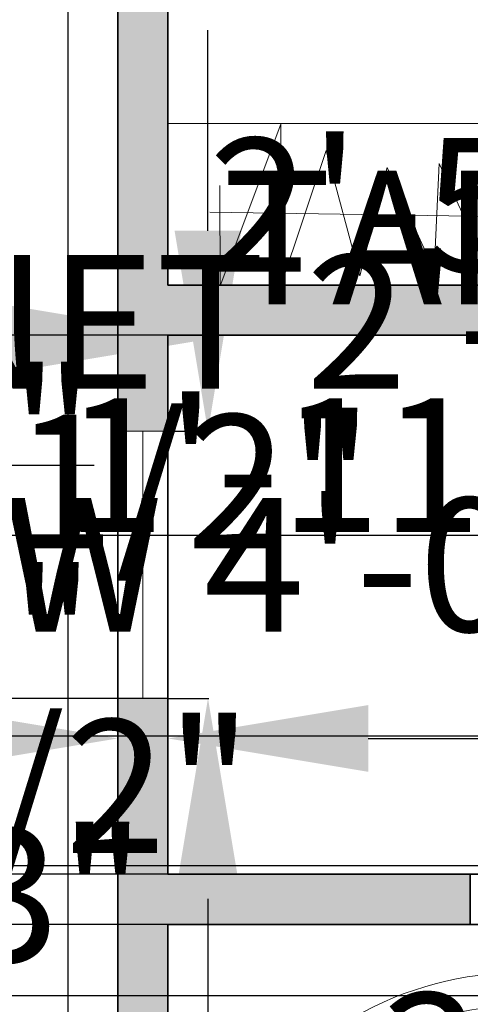
# Model space of a CAD drawing. Units: inches. Extents: x 2838 to 4029, y 1041 to 1915.
# Tile 5 of 16: x 3250 to 3331, y 1377 to 1554. Entities that reach past the tile are written whole.
import ezdxf

# ---------------------------------------------------------------- set-up
doc = ezdxf.new("R2010")
doc.units = ezdxf.units.IN
doc.header["$MEASUREMENT"] = 0
for name, color, linetype, lineweight in [('A-ANNO-DIMS', 2, 'Continuous', 18), ('A-FLOR', 7, 'Continuous', 25), ('A-FLOR-CASE', 8, 'Continuous', 18), ('A-FURN', 8, 'Continuous', 18), ('A-GLAZ', 4, 'Continuous', 18), ('A-WALL', 7, 'Continuous', 35), ('A-WALL-PATT', 252, 'Continuous', 13)]:
    doc.layers.add(name, color=color, linetype=linetype, lineweight=lineweight)
doc.styles.get("Standard").update_dxf_attribs({"font": 'arial.ttf'})
doc.dimstyles.get("Standard").update_dxf_attribs({"dimtxt": 24, "dimasz": 36, "dimexe": 0.18, "dimexo": 0.0625, "dimgap": 0.09, "dimtad": 0, "dimtih": 1, "dimtoh": 1, "dimdec": 0, "dimzin": 0, "dimdsep": 46, "dimlunit": 3, "dimtxsty": 'Standard', "dimcen": 0.09, "dimadec": 0, "dimazin": 0, "dimtfac": 1, "dimtdec": 0, "dimtofl": 0, "dimtmove": 0, "dimatfit": 3, "dimfxl": 1, "dimtolj": 1, "dimtzin": 0, "dimarcsym": 0})

# ---------------------------------------------------------------- blocks, each defined once
blk = doc.blocks.new('Sofa - Roundback Loveseat 5 ft.')
for p, q in [((0, -32.44198), (0, -5.99998)), ((-24, -33.99998), (-24, -11.46958)), ((24.00004, -33.99998), (24.00004, -11.46958)), ((-23.9998, -13.38178), (23.99986, -13.38178)), ((-24, -32.44198), (24.00004, -32.44198))]:
    blk.add_line(p, q)
for points in [[(-24, -33.99998), (-30, -33.99998), (-30, -7.99998)], [(30.00004, -7.99998), (30.00004, -33.99998), (24.00004, -33.99998)]]:
    blk.add_lwpolyline(points)
for centre, radius, start, end in [((0, -60.24998), 60.24998, 60.13715, 119.8628), ((0, -61.38438), 55.38444, 64.32083, 115.6792)]:
    blk.add_arc(centre, radius, start, end)
blk = doc.blocks.new('WIN-48')
blk.add_line((4.5, 48), (4.5, 0))
blk.add_lwpolyline([(0, 48), (9, 48), (9, 0), (0, 0)], close=True)
blk = doc.blocks.new('WARDROBE-RAIL')
for p, q in [((1.86, 0), (12.76, 29.05)), ((12.76, 29.05), (12.76, 0)), ((12.76, 0), (20.9, 24.31)), ((20.9, 24.31), (26.94, 1.83)), ((26.94, 1.83), (31.9, 21.29)), ((31.9, 21.29), (40.3, 2.75)), ((40.3, 2.75), (41.22, 21.97)), ((41.22, 21.97), (49.7, 3.76)), ((1.8, 18), (1.86, 0)), ((49.7, 3.76), (51.56, 19.2)), ((51.56, 19.2), (58.03, 7.54)), ((58.03, 7.54), (58.45, 19.29)), ((58.45, 19.29), (63.49, 12.24)), ((63.49, 12.24), (0, 13.24)), ((0, 13.24), (63.49, 12.24))]:
    blk.add_line(p, q)
blk = doc.blocks.new('*D25')
at = {"layer": 'A-ANNO-DIMS', "color": 0, "lineweight": -2, "transparency": 16777216}
for p, q in [((3283.93, 1516.17), (3283.93, 1552.17)), ((3276.79, 1480.17), (3284.11, 1480.17)), ((3276.79, 1432.17), (3284.11, 1432.17)), ((3283.93, 1396.17), (3283.93, 1360.17))]:
    blk.add_line(p, q, dxfattribs=at)
at = {"layer": 'A-ANNO-DIMS', "color": 0, "transparency": 16777216}
for points in [[(3277.93, 1516.17), (3289.93, 1516.17), (3283.93, 1480.17)], [(3277.93, 1396.17), (3289.93, 1396.17), (3283.93, 1432.17)]]:
    blk.add_solid(points, dxfattribs=at)
at = {"layer": 'Defpoints', "color": 0, "transparency": 16777216}
for p in [(3276.73, 1480.17), (3283.93, 1480.17), (3276.73, 1432.17)]:
    blk.add_point(p, dxfattribs=at)
at = {"layer": 'A-ANNO-DIMS', "color": 0, "transparency": 16777216, "insert": (3283.93, 1456.17), "char_height": 24, "attachment_point": 5}
blk.add_mtext('\\A1;WINDOW 4\'-0" TYP.', dxfattribs=at)
blk = doc.blocks.new('*D26')
at = {"layer": 'A-ANNO-DIMS', "color": 0, "lineweight": -2, "transparency": 16777216}
for p, q in [((3267.73, 1432.1), (3267.73, 1424.79)), ((3276.73, 1432.1), (3276.73, 1424.79)), ((3231.73, 1424.97), (3195.73, 1424.97)), ((3312.73, 1424.97), (3348.73, 1424.97))]:
    blk.add_line(p, q, dxfattribs=at)
at = {"layer": 'A-ANNO-DIMS', "color": 0, "transparency": 16777216}
for points in [[(3231.73, 1430.97), (3231.73, 1418.97), (3267.73, 1424.97)], [(3312.73, 1430.97), (3312.73, 1418.97), (3276.73, 1424.97)]]:
    blk.add_solid(points, dxfattribs=at)
at = {"layer": 'Defpoints', "color": 0, "transparency": 16777216}
for p in [(3267.73, 1432.17), (3276.73, 1432.17), (3276.73, 1424.97)]:
    blk.add_point(p, dxfattribs=at)
at = {"layer": 'A-ANNO-DIMS', "color": 0, "transparency": 16777216, "insert": (3421.97, 1424.97), "char_height": 24, "attachment_point": 5}
blk.add_mtext('\\A1;0\'-9" TYP.', dxfattribs=at)
blk = doc.blocks.new('*D30')
at = {"layer": 'A-ANNO-DIMS', "color": 0, "lineweight": -2, "transparency": 16777216}
for p, q in [((3379.15, 1421.58), (3379.15, 1457.58)), ((3370.21, 1385.58), (3379.33, 1385.58)), ((3370.21, 1348.91), (3379.33, 1348.91)), ((3379.15, 1312.91), (3379.15, 1276.91))]:
    blk.add_line(p, q, dxfattribs=at)
at = {"layer": 'A-ANNO-DIMS', "color": 0, "transparency": 16777216}
for points in [[(3373.15, 1421.58), (3385.15, 1421.58), (3379.15, 1385.58)], [(3373.15, 1312.91), (3385.15, 1312.91), (3379.15, 1348.91)]]:
    blk.add_solid(points, dxfattribs=at)
at = {"layer": 'Defpoints', "color": 0, "transparency": 16777216}
for p in [(3370.15, 1385.58), (3379.15, 1385.58), (3370.15, 1348.91)]:
    blk.add_point(p, dxfattribs=at)
at = {"layer": 'A-ANNO-DIMS', "color": 0, "transparency": 16777216, "insert": (3379.15, 1367.25), "char_height": 24, "attachment_point": 5}
blk.add_mtext('\\A1;3\'-0 1/2"', dxfattribs=at)
blk = doc.blocks.new('*D35')
at = {"layer": 'A-ANNO-DIMS', "color": 0, "lineweight": -2, "transparency": 16777216}
for p, q in [((3480.45, 1632.93), (3480.45, 1668.93)), ((3481.89, 1596.93), (3480.27, 1596.93)), ((3481.89, 1586.93), (3480.27, 1586.93)), ((3480.45, 1550.93), (3480.45, 1514.93)), ((3480.45, 1514.93), (3444.45, 1514.93))]:
    blk.add_line(p, q, dxfattribs=at)
at = {"layer": 'A-ANNO-DIMS', "color": 0, "transparency": 16777216}
for points in [[(3474.45, 1632.93), (3486.45, 1632.93), (3480.45, 1596.93)], [(3474.45, 1550.93), (3486.45, 1550.93), (3480.45, 1586.93)]]:
    blk.add_solid(points, dxfattribs=at)
at = {"layer": 'Defpoints', "color": 0, "transparency": 16777216}
for p in [(3481.95, 1596.93), (3480.45, 1586.93), (3481.95, 1586.93)]:
    blk.add_point(p, dxfattribs=at)
at = {"layer": 'A-ANNO-DIMS', "color": 0, "transparency": 16777216, "insert": (3365.58, 1514.93), "char_height": 24, "attachment_point": 5}
blk.add_mtext('\\A1;TAP 0\'-10"', dxfattribs=at)
blk = doc.blocks.new('*D38')
at = {"layer": 'A-ANNO-DIMS', "color": 0, "lineweight": -2, "transparency": 16777216}
for p, q in [((3368.73, 1671.36), (3368.73, 1707.36)), ((3356.79, 1635.36), (3368.91, 1635.36)), ((3356.79, 1575.36), (3368.91, 1575.36)), ((3368.73, 1539.36), (3368.73, 1503.36))]:
    blk.add_line(p, q, dxfattribs=at)
at = {"layer": 'A-ANNO-DIMS', "color": 0, "transparency": 16777216}
for points in [[(3362.73, 1671.36), (3374.73, 1671.36), (3368.73, 1635.36)], [(3362.73, 1539.36), (3374.73, 1539.36), (3368.73, 1575.36)]]:
    blk.add_solid(points, dxfattribs=at)
at = {"layer": 'Defpoints', "color": 0, "transparency": 16777216}
for p in [(3356.73, 1635.36), (3368.73, 1635.36), (3356.73, 1575.36)]:
    blk.add_point(p, dxfattribs=at)
at = {"layer": 'A-ANNO-DIMS', "color": 0, "transparency": 16777216, "insert": (3368.73, 1605.36), "char_height": 24, "attachment_point": 5}
blk.add_mtext('\\A1;5\'-0" TYP.', dxfattribs=at)
blk = doc.blocks.new('*D41')
at = {"layer": 'A-ANNO-DIMS', "color": 0, "lineweight": -2, "transparency": 16777216}
for p, q in [((3284.24, 1506.2), (3284.24, 1496.56)), ((3347.73, 1506.2), (3347.73, 1496.56)), ((3248.24, 1496.74), (3212.24, 1496.74)), ((3383.73, 1496.74), (3419.73, 1496.74))]:
    blk.add_line(p, q, dxfattribs=at)
at = {"layer": 'A-ANNO-DIMS', "color": 0, "transparency": 16777216}
for points in [[(3248.24, 1502.74), (3248.24, 1490.74), (3284.24, 1496.74)], [(3383.73, 1502.74), (3383.73, 1490.74), (3347.73, 1496.74)]]:
    blk.add_solid(points, dxfattribs=at)
at = {"layer": 'Defpoints', "color": 0, "transparency": 16777216}
for p in [(3284.24, 1506.26), (3347.73, 1506.26), (3347.73, 1496.74)]:
    blk.add_point(p, dxfattribs=at)
at = {"layer": 'A-ANNO-DIMS', "color": 0, "transparency": 16777216, "insert": (3624.81, 1496.74), "char_height": 24, "attachment_point": 5}
blk.add_mtext('\\A1;WARDROBE 5\'-3 1/2" TYP.', dxfattribs=at)
blk = doc.blocks.new('*D42')
at = {"layer": 'A-ANNO-DIMS', "color": 0, "lineweight": -2, "transparency": 16777216}
for p, q in [((3357.26, 1571.32), (3357.26, 1607.32)), ((3347.8, 1535.32), (3357.44, 1535.32)), ((3347.8, 1506.26), (3357.44, 1506.26)), ((3357.26, 1470.26), (3357.26, 1434.26))]:
    blk.add_line(p, q, dxfattribs=at)
at = {"layer": 'A-ANNO-DIMS', "color": 0, "transparency": 16777216}
for points in [[(3351.26, 1571.32), (3363.26, 1571.32), (3357.26, 1535.32)], [(3351.26, 1470.26), (3363.26, 1470.26), (3357.26, 1506.26)]]:
    blk.add_solid(points, dxfattribs=at)
at = {"layer": 'Defpoints', "color": 0, "transparency": 16777216}
for p in [(3347.73, 1535.32), (3357.26, 1535.32), (3347.73, 1506.26)]:
    blk.add_point(p, dxfattribs=at)
at = {"layer": 'A-ANNO-DIMS', "color": 0, "transparency": 16777216, "insert": (3357.26, 1520.79), "char_height": 24, "attachment_point": 5}
blk.add_mtext('\\A1;2\'-5" TYP.', dxfattribs=at)
blk = doc.blocks.new('*D55')
at = {"layer": 'A-ANNO-DIMS', "color": 0, "lineweight": -2, "transparency": 16777216}
for p, q in [((3491.76, 1499.78), (3455.76, 1499.78)), ((3527.76, 1494.67), (3527.76, 1499.96)), ((3562.26, 1494.67), (3562.26, 1499.96)), ((3598.26, 1499.78), (3634.26, 1499.78))]:
    blk.add_line(p, q, dxfattribs=at)
at = {"layer": 'A-ANNO-DIMS', "color": 0, "transparency": 16777216}
for points in [[(3491.76, 1505.78), (3491.76, 1493.78), (3527.76, 1499.78)], [(3598.26, 1505.78), (3598.26, 1493.78), (3562.26, 1499.78)]]:
    blk.add_solid(points, dxfattribs=at)
at = {"layer": 'Defpoints', "color": 0, "transparency": 16777216}
for p in [(3527.76, 1499.78), (3527.76, 1494.6), (3562.26, 1494.6)]:
    blk.add_point(p, dxfattribs=at)
at = {"layer": 'A-ANNO-DIMS', "color": 0, "transparency": 16777216, "insert": (3260.33, 1499.78), "char_height": 24, "attachment_point": 5}
blk.add_mtext('\\A1;BASE CABINET 2\'-10 1/2"', dxfattribs=at)
blk = doc.blocks.new('*D59')
at = {"layer": 'A-ANNO-DIMS', "color": 0, "lineweight": -2, "transparency": 16777216}
for p, q in [((3055.85, 1478.53), (3055.85, 1470.96)), ((3117.35, 1478.53), (3117.35, 1470.96)), ((3019.85, 1471.14), (2983.85, 1471.14)), ((3153.35, 1471.14), (3189.35, 1471.14))]:
    blk.add_line(p, q, dxfattribs=at)
at = {"layer": 'A-ANNO-DIMS', "color": 0, "transparency": 16777216}
for points in [[(3019.85, 1477.14), (3019.85, 1465.14), (3055.85, 1471.14)], [(3153.35, 1477.14), (3153.35, 1465.14), (3117.35, 1471.14)]]:
    blk.add_solid(points, dxfattribs=at)
at = {"layer": 'Defpoints', "color": 0, "transparency": 16777216}
for p in [(3055.85, 1478.59), (3117.35, 1478.59), (3117.35, 1471.14)]:
    blk.add_point(p, dxfattribs=at)
at = {"layer": 'A-ANNO-DIMS', "color": 0, "transparency": 16777216, "insert": (3249.3, 1471.14), "char_height": 24, "attachment_point": 5}
blk.add_mtext('\\A1;5\'-1 1/2"', dxfattribs=at)
blk = doc.blocks.new('*D67')
at = {"layer": 'A-ANNO-DIMS', "color": 0, "lineweight": -2, "transparency": 16777216}
for p, q in [((3258.67, 1680.3), (3227.33, 1680.3)), ((3227.51, 1644.3), (3227.51, 1409.15)), ((3227.51, 1149.3), (3227.51, 1384.45)), ((3329.6, 1113.3), (3227.33, 1113.3))]:
    blk.add_line(p, q, dxfattribs=at)
at = {"layer": 'A-ANNO-DIMS', "color": 0, "transparency": 16777216}
for points in [[(3221.51, 1644.3), (3233.51, 1644.3), (3227.51, 1680.3)], [(3221.51, 1149.3), (3233.51, 1149.3), (3227.51, 1113.3)]]:
    blk.add_solid(points, dxfattribs=at)
at = {"layer": 'Defpoints', "color": 0, "transparency": 16777216}
for p in [(3227.51, 1680.3), (3258.73, 1680.3), (3329.66, 1113.3)]:
    blk.add_point(p, dxfattribs=at)
at = {"layer": 'A-ANNO-DIMS', "color": 0, "transparency": 16777216, "insert": (3227.51, 1396.8), "char_height": 24, "attachment_point": 5}
blk.add_mtext('\\A1;47\'-3"', dxfattribs=at)
blk = doc.blocks.new('*D76')
at = {"layer": 'A-ANNO-DIMS', "color": 0, "lineweight": -2, "transparency": 16777216}
for p, q in [((3276.67, 1391.57), (3227.33, 1391.57)), ((3227.51, 1355.57), (3227.51, 1303.94)), ((3227.51, 1227.3), (3227.51, 1278.94)), ((3267.67, 1191.3), (3227.33, 1191.3))]:
    blk.add_line(p, q, dxfattribs=at)
at = {"layer": 'A-ANNO-DIMS', "color": 0, "transparency": 16777216}
for points in [[(3221.51, 1355.57), (3233.51, 1355.57), (3227.51, 1391.57)], [(3221.51, 1227.3), (3233.51, 1227.3), (3227.51, 1191.3)]]:
    blk.add_solid(points, dxfattribs=at)
at = {"layer": 'Defpoints', "color": 0, "transparency": 16777216}
for p in [(3227.51, 1391.57), (3276.73, 1391.57), (3267.73, 1191.3)]:
    blk.add_point(p, dxfattribs=at)
at = {"layer": 'A-ANNO-DIMS', "color": 0, "transparency": 16777216, "insert": (3227.51, 1291.44), "char_height": 24, "attachment_point": 5}
blk.add_mtext('\\A1;16\'-8 1/2"', dxfattribs=at)
blk = doc.blocks.new('*D77')
at = {"layer": 'A-ANNO-DIMS', "color": 0, "lineweight": -2, "transparency": 16777216}
for p, q in [((3267.67, 1671.3), (3227.33, 1671.3)), ((3227.51, 1635.3), (3227.51, 1596.69)), ((3227.51, 1533.39), (3227.51, 1572)), ((3276.67, 1497.39), (3227.33, 1497.39))]:
    blk.add_line(p, q, dxfattribs=at)
at = {"layer": 'A-ANNO-DIMS', "color": 0, "transparency": 16777216}
for points in [[(3221.51, 1635.3), (3233.51, 1635.3), (3227.51, 1671.3)], [(3221.51, 1533.39), (3233.51, 1533.39), (3227.51, 1497.39)]]:
    blk.add_solid(points, dxfattribs=at)
at = {"layer": 'Defpoints', "color": 0, "transparency": 16777216}
for p in [(3227.51, 1671.3), (3267.73, 1671.3), (3276.73, 1497.39)]:
    blk.add_point(p, dxfattribs=at)
at = {"layer": 'A-ANNO-DIMS', "color": 0, "transparency": 16777216, "insert": (3227.51, 1584.35), "char_height": 24, "attachment_point": 5}
blk.add_mtext('\\A1;14\'-6"', dxfattribs=at)
blk = doc.blocks.new('*D87')
at = {"layer": 'A-ANNO-DIMS', "color": 0, "lineweight": -2, "transparency": 16777216}
for p, q in [((3227.506626, 1497.394218), (3227.506626, 1533.394218)), ((3513.669126, 1461.394218), (3227.326626, 1461.394218)), ((3513.669126, 1425.394218), (3227.326626, 1425.394218)), ((3227.506626, 1389.394218), (3227.506626, 1353.394218))]:
    blk.add_line(p, q, dxfattribs=at)
at = {"layer": 'A-ANNO-DIMS', "color": 0, "transparency": 16777216}
for points in [[(3221.506626, 1497.394218), (3233.506626, 1497.394218), (3227.506626, 1461.394218)], [(3221.506626, 1389.394218), (3233.506626, 1389.394218), (3227.506626, 1425.394218)]]:
    blk.add_solid(points, dxfattribs=at)
at = {"layer": 'Defpoints', "color": 0, "transparency": 16777216}
for p in [(3227.506626, 1461.394218), (3513.731626, 1461.394218), (3513.731626, 1425.394218)]:
    blk.add_point(p, dxfattribs=at)
at = {"layer": 'A-ANNO-DIMS', "color": 0, "transparency": 16777216, "insert": (3227.506626, 1443.394218), "char_height": 24, "attachment_point": 5}
blk.add_mtext('\\A1;3\'-0"', dxfattribs=at)
blk = doc.blocks.new('*D91')
at = {"layer": 'A-ANNO-DIMS', "color": 0, "lineweight": -2, "transparency": 16777216}
for p, q in [((3227.506626, 1533.394218), (3227.506626, 1569.394218)), ((3522.669126, 1497.394218), (3227.326626, 1497.394218)), ((3522.669126, 1461.394218), (3227.326626, 1461.394218)), ((3227.506626, 1425.394218), (3227.506626, 1389.394218))]:
    blk.add_line(p, q, dxfattribs=at)
at = {"layer": 'A-ANNO-DIMS', "color": 0, "transparency": 16777216}
for points in [[(3221.506626, 1533.394218), (3233.506626, 1533.394218), (3227.506626, 1497.394218)], [(3221.506626, 1425.394218), (3233.506626, 1425.394218), (3227.506626, 1461.394218)]]:
    blk.add_solid(points, dxfattribs=at)
at = {"layer": 'Defpoints', "color": 0, "transparency": 16777216}
for p in [(3522.731626, 1497.394218), (3227.506626, 1461.394218), (3522.731626, 1461.394218)]:
    blk.add_point(p, dxfattribs=at)
at = {"layer": 'A-ANNO-DIMS', "color": 0, "transparency": 16777216, "insert": (3227.506626, 1479.394218), "char_height": 24, "attachment_point": 5}
blk.add_mtext('\\A1;3\'-0"', dxfattribs=at)
blk = doc.blocks.new('*D93')
at = {"layer": 'A-ANNO-DIMS', "color": 0, "lineweight": -2, "transparency": 16777216}
for p, q in [((3227.51, 1438.06), (3227.51, 1474.06)), ((3227.51, 1474.06), (3263.51, 1474.06)), ((3522.67, 1402.06), (3227.33, 1402.06)), ((3522.67, 1378.73), (3227.33, 1378.73)), ((3227.51, 1342.73), (3227.51, 1306.73))]:
    blk.add_line(p, q, dxfattribs=at)
at = {"layer": 'A-ANNO-DIMS', "color": 0, "transparency": 16777216}
for points in [[(3221.51, 1438.06), (3233.51, 1438.06), (3227.51, 1402.06)], [(3221.51, 1342.73), (3233.51, 1342.73), (3227.51, 1378.73)]]:
    blk.add_solid(points, dxfattribs=at)
at = {"layer": 'Defpoints', "color": 0, "transparency": 16777216}
for p in [(3227.51, 1402.06), (3522.73, 1402.06), (3522.73, 1378.73)]:
    blk.add_point(p, dxfattribs=at)
at = {"layer": 'A-ANNO-DIMS', "color": 0, "transparency": 16777216, "insert": (3331.65, 1474.06), "char_height": 24, "attachment_point": 5}
blk.add_mtext('\\A1;1\'-11 1/2"', dxfattribs=at)
blk = doc.blocks.new('*D95')
at = {"layer": 'A-ANNO-DIMS', "color": 0, "lineweight": -2, "transparency": 16777216}
for p, q in [((3227.51, 1468.17), (3227.51, 1504.17)), ((3276.67, 1432.17), (3227.33, 1432.17)), ((3276.67, 1400.57), (3227.33, 1400.57)), ((3227.51, 1364.57), (3227.51, 1328.57))]:
    blk.add_line(p, q, dxfattribs=at)
at = {"layer": 'A-ANNO-DIMS', "color": 0, "transparency": 16777216}
for points in [[(3221.51, 1468.17), (3233.51, 1468.17), (3227.51, 1432.17)], [(3221.51, 1364.57), (3233.51, 1364.57), (3227.51, 1400.57)]]:
    blk.add_solid(points, dxfattribs=at)
at = {"layer": 'Defpoints', "color": 0, "transparency": 16777216}
for p in [(3227.51, 1432.17), (3276.73, 1432.17), (3276.73, 1400.57)]:
    blk.add_point(p, dxfattribs=at)
at = {"layer": 'A-ANNO-DIMS', "color": 0, "transparency": 16777216, "insert": (3227.51, 1416.37), "char_height": 24, "attachment_point": 5}
blk.add_mtext('\\A1;2\'-7 1/2"', dxfattribs=at)
blk = doc.blocks.new('*D103')
at = {"layer": 'A-ANNO-DIMS', "color": 0, "lineweight": -2, "transparency": 16777216}
for p, q in [((3227.51, 1628.55), (3227.51, 1664.55)), ((3227.51, 1664.55), (3263.51, 1664.55)), ((3469.64, 1592.55), (3227.33, 1592.55)), ((3441.67, 1578.3), (3227.33, 1578.3)), ((3227.51, 1542.3), (3227.51, 1506.3))]:
    blk.add_line(p, q, dxfattribs=at)
at = {"layer": 'A-ANNO-DIMS', "color": 0, "transparency": 16777216}
for points in [[(3221.51, 1628.55), (3233.51, 1628.55), (3227.51, 1592.55)], [(3221.51, 1542.3), (3233.51, 1542.3), (3227.51, 1578.3)]]:
    blk.add_solid(points, dxfattribs=at)
at = {"layer": 'Defpoints', "color": 0, "transparency": 16777216}
for p in [(3227.51, 1592.55), (3469.7, 1592.55), (3441.73, 1578.3)]:
    blk.add_point(p, dxfattribs=at)
at = {"layer": 'A-ANNO-DIMS', "color": 0, "transparency": 16777216, "insert": (3322.33, 1664.55), "char_height": 24, "attachment_point": 5}
blk.add_mtext('\\A1;1\'-2 1/2"', dxfattribs=at)

msp = doc.modelspace()

# ---------------------------------------------------------------- hatches: boundary and pattern name
at = {"layer": 'A-WALL-PATT'}
h = msp.add_hatch(color=256, dxfattribs=at)
h.dxf.hatch_style = 1
h.paths.add_polyline_path([(3405.73, 1506.39), (3297.05, 1506.39), (3297.01, 1506.26), (3297.01, 1506.39), (3286.16, 1506.39), (3286.11, 1506.26), (3286.11, 1506.39), (3276.73, 1506.39), (3276.73, 1535.45), (3276.73, 1662.3), (3312.91, 1662.3), (3312.91, 1671.3), (3267.73, 1671.3), (3267.73, 1480.17), (3276.73, 1480.17), (3276.73, 1497.39), (3405.73, 1497.39)])
h = msp.add_hatch(color=256, dxfattribs=at)
h.dxf.hatch_style = 1
h.paths.add_polyline_path([(3427.52, 1671.3), (3360.91, 1671.3), (3360.91, 1662.3), (3396.73, 1662.3), (3396.73, 1554.39), (3397.12, 1554.39, -0.007312), (3398.53, 1554.41), (3405.73, 1554.41), (3405.73, 1662.3), (3427.52, 1662.3)])
h.paths.add_polyline_path([(3546.42, 1671.3), (3451.52, 1671.3), (3451.52, 1662.3), (3489.73, 1662.3), (3489.73, 1592.86, -0.016107), (3489.73, 1591.9), (3489.73, 1578.3), (3441.73, 1578.3), (3441.73, 1569.3), (3489.73, 1569.3), (3489.73, 1554.41), (3498.73, 1554.41), (3498.73, 1662.3), (3546.42, 1662.3)])
h.paths.add_polyline_path([(3627.73, 1671.3), (3594.42, 1671.3), (3594.42, 1662.3), (3618.73, 1662.3), (3618.73, 1634.03), (3627.73, 1634.03)])
h.paths.add_polyline_path([(3627.73, 1586.03), (3618.73, 1586.03), (3618.73, 1506.39), (3545.12, 1506.39), (3489.73, 1506.39), (3489.73, 1497.39), (3513.73, 1497.39), (3618.73, 1497.39), (3618.73, 1469.85), (3627.73, 1469.85)])
h.paths.add_polyline_path([(3627.73, 1421.85), (3618.73, 1421.85), (3618.73, 1378.73), (3522.73, 1378.73), (3513.73, 1378.73), (3461.04, 1378.73), (3461.04, 1369.73), (3513.73, 1369.73), (3618.73, 1369.73), (3618.73, 1320.94), (3627.73, 1320.94)])
h.paths.add_polyline_path([(3627.73, 1272.94), (3618.73, 1272.94), (3618.73, 1200.3), (3599.07, 1200.3), (3599.07, 1191.3), (3627.73, 1191.3)])
h.paths.add_polyline_path([(3551.07, 1200.3), (3510.18, 1200.3), (3510.18, 1191.3), (3551.07, 1191.3)])
h.paths.add_polyline_path([(3486.18, 1200.3), (3461.04, 1200.3), (3461.04, 1398.25), (3454.63, 1398.25), (3454.63, 1200.3), (3432.45, 1200.3), (3432.45, 1191.3), (3486.18, 1191.3)])
h.paths.add_polyline_path([(3300.73, 1200.3), (3276.73, 1200.3), (3276.73, 1391.57), (3331.05, 1391.57), (3331.05, 1400.57), (3276.73, 1400.57), (3276.73, 1432.17), (3267.73, 1432.17), (3267.73, 1191.3), (3300.73, 1191.3)])

# ---------------------------------------------------------------- linework, layer by layer
at = {"layer": 'A-FLOR'}
msp.add_lwpolyline([(3527.95, 1182.3), (3636.73, 1182.3), (3636.73, 1680.3), (3258.73, 1680.3), (3258.73, 1182.3), (3267.73, 1182.3)], dxfattribs=at)
at = {"layer": 'A-FLOR-CASE'}
msp.add_lwpolyline([(3276.73, 1535.45), (3350.34, 1535.45), (3350.34, 1506.39), (3276.73, 1506.39)], close=True, dxfattribs=at)
at = {"layer": 'A-WALL'}
for p, q in [((3267.73, 1671.3), (3267.73, 1191.3)), ((3276.73, 1662.3), (3276.73, 1506.39)), ((3276.73, 1506.39), (3276.73, 1662.3)), ((3405.73, 1506.39), (3276.73, 1506.39)), ((3405.73, 1506.39), (3276.73, 1506.39)), ((3405.73, 1497.39), (3276.73, 1497.39)), ((3276.73, 1497.39), (3276.73, 1400.57)), ((3276.73, 1480.17), (3276.73, 1497.39)), ((3276.73, 1497.39), (3405.73, 1497.39)), ((3276.73, 1432.17), (3276.73, 1480.17)), ((3276.73, 1400.57), (3276.73, 1432.17)), ((3379.05, 1400.57), (3276.73, 1400.57)), ((3379.05, 1400.57), (3276.73, 1400.57)), ((3331.05, 1400.57), (3276.73, 1400.57)), ((3331.05, 1391.57), (3331.05, 1400.57)), ((3379.05, 1391.57), (3276.73, 1391.57)), ((3379.05, 1391.57), (3276.73, 1391.57)), ((3276.73, 1391.57), (3276.73, 1200.3)), ((3276.73, 1200.3), (3276.73, 1391.57)), ((3276.73, 1391.57), (3331.05, 1391.57))]:
    msp.add_line(p, q, dxfattribs=at)
msp.add_lwpolyline([(3372.73, 1191.3), (3627.73, 1191.3), (3627.73, 1671.3), (3267.73, 1671.3), (3267.73, 1191.3), (3300.73, 1191.3)], dxfattribs=at)

# ---------------------------------------------------------------- block references
at = {"layer": 'A-FLOR-CASE'}
msp.add_blockref('WARDROBE-RAIL', (3284.24, 1506.26), dxfattribs=at)
at = {"layer": 'A-FURN'}
msp.add_blockref('Sofa - Roundback Loveseat 5 ft.', (3340.15, 1382.91), dxfattribs=at)
at = {"layer": 'A-GLAZ'}
msp.add_blockref('WIN-48', (3267.73, 1432.17), dxfattribs=at)

# ---------------------------------------------------------------- dimensions: what is measured, and where the dimension line sits
at = {"layer": 'A-ANNO-DIMS'}
for base, p1, p2, angle, text, picture, middle in [((3368.73, 1635.36), (3356.73, 1575.36), (3356.73, 1635.36), 90, '<> TYP.', '*D38', (3368.73, 1605.36)), ((3480.45, 1586.93), (3481.95, 1596.93), (3481.95, 1586.93), 270, 'TAP <>', '*D35', (3365.58, 1514.93)), ((3357.26, 1535.32), (3347.73, 1506.26), (3347.73, 1535.32), 90, '<> TYP.', '*D42', (3357.26, 1520.79)), ((3527.76, 1499.78), (3562.26, 1494.6), (3527.76, 1494.6), 180, 'BASE CABINET <>', '*D55', (3260.33, 1499.78)), ((3283.93, 1480.17), (3276.73, 1432.17), (3276.73, 1480.17), 90, 'WINDOW <> TYP.', '*D25', (3283.93, 1456.17))]:
    dim = msp.add_linear_dim(base=base, p1=p1, p2=p2, angle=angle, text=text, dimstyle='Standard', override={"dimdec": 1, "dimlfac": 1, "dimrnd": 0, "dimzin": 1, "dimdsep": 46, "dimlunit": 4, "dimfrac": 2}, dxfattribs=at)
    dim.commit()
    dim.dimension.update_dxf_attribs({"geometry": picture, "text_midpoint": middle})
for base, p1, p2, picture, middle in [((3227.5066, 1592.5486), (3441.7316, 1578.2973), (3469.6999, 1592.5486), '*D103', (3322.3279, 1664.5486)), ((3227.51, 1680.3), (3329.66, 1113.3), (3258.73, 1680.3), '*D67', (3227.51, 1396.8)), ((3227.51, 1671.3), (3276.73, 1497.39), (3267.73, 1671.3), '*D77', (3227.51, 1584.35)), ((3227.51, 1461.39), (3522.73, 1497.39), (3522.73, 1461.39), '*D91', (3227.51, 1479.39)), ((3227.51, 1461.39), (3513.73, 1425.39), (3513.73, 1461.39), '*D87', (3227.51, 1443.39)), ((3227.51, 1402.06), (3522.73, 1378.73), (3522.73, 1402.06), '*D93', (3331.65, 1474.06)), ((3227.51, 1432.17), (3276.73, 1400.57), (3276.73, 1432.17), '*D95', (3227.51, 1416.37)), ((3379.15, 1385.58), (3370.15, 1348.91), (3370.15, 1385.58), '*D30', (3379.15, 1367.25)), ((3227.51, 1391.57), (3267.73, 1191.3), (3276.73, 1391.57), '*D76', (3227.51, 1291.44))]:
    dim = msp.add_linear_dim(base=base, p1=p1, p2=p2, angle=90, dimstyle='Standard', override={"dimdec": 1, "dimlfac": 1, "dimrnd": 0, "dimzin": 1, "dimdsep": 46, "dimlunit": 4, "dimfrac": 2}, dxfattribs=at)
    dim.commit()
    dim.dimension.update_dxf_attribs({"geometry": picture, "text_midpoint": middle})
for base, p1, p2, text, picture, middle in [((3347.73, 1496.74), (3284.24, 1506.26), (3347.73, 1506.26), 'WARDROBE <> TYP.', '*D41', (3624.81, 1496.74)), ((3276.73, 1424.97), (3267.73, 1432.17), (3276.73, 1432.17), '<> TYP.', '*D26', (3421.97, 1424.97))]:
    dim = msp.add_linear_dim(base=base, p1=p1, p2=p2, text=text, dimstyle='Standard', override={"dimdec": 1, "dimlfac": 1, "dimrnd": 0, "dimzin": 1, "dimdsep": 46, "dimlunit": 4, "dimfrac": 2}, dxfattribs=at)
    dim.commit()
    dim.dimension.update_dxf_attribs({"geometry": picture, "text_midpoint": middle})
dim = msp.add_linear_dim(base=(3117.35, 1471.14), p1=(3055.85, 1478.59), p2=(3117.35, 1478.59), dimstyle='Standard', override={"dimdec": 1, "dimlfac": 1, "dimrnd": 0, "dimzin": 1, "dimdsep": 46, "dimlunit": 4, "dimfrac": 2}, dxfattribs=at)
dim.commit()
dim.dimension.update_dxf_attribs({"geometry": '*D59', "text_midpoint": (3249.3, 1471.14)})

doc.saveas('drawing.dxf')
